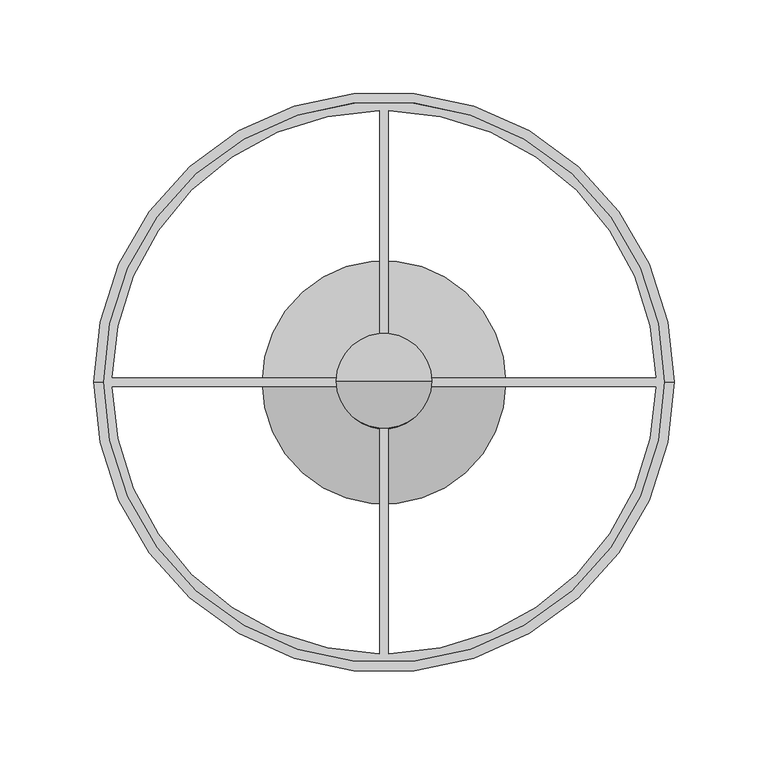
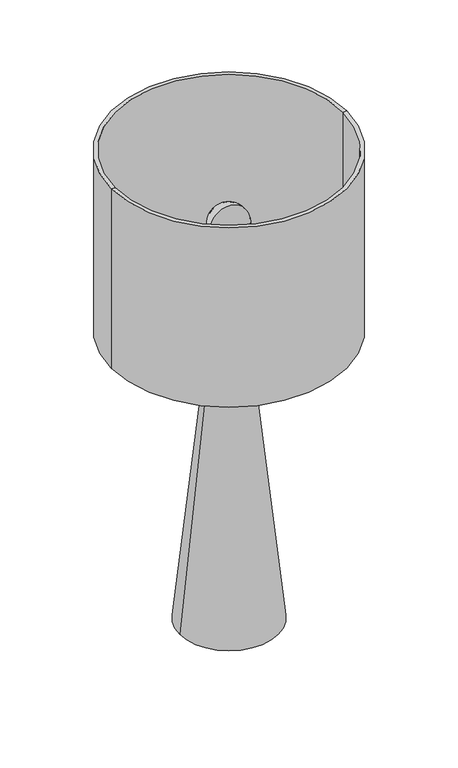
"""IFC4 building model written with IfcOpenShell, lengths in millimetres: furniture geometry."""

from ifc_helpers import new_model, si_unit, point, frame, frame_2d, origin, place, context, project, spatial, polyline, circle_curve, ellipse_curve, trimmed, segment, composite_curve, outline, extrude, source, transform, mapped, element, save
from ifc_brep_helpers import plane_surface, cylinder_surface, revolved_surface, advanced_brep


def furniture_2a5d2cbe(model_context):
    return source(origin(), model_context, "Body", "SolidModel", [
        advanced_brep(
        [(239.3621376, 642.8775263, 489.7915015), (258.4121376, 642.8775263, 489.7915015), (258.4121376, 642.8775263, 478.3555771), (239.3621376, 642.8775263, 478.3555771), (248.8871376, 642.8775263, 489.7915015), (245.7708139, 642.8775263, 472.622676), (252.0034612, 642.8775263, 472.622676), (248.8871376, 642.8775263, 472.622676), (244.5637531, 642.8775263, 474.7133667), (253.2105221, 642.8775263, 474.7133667)],
        [
            (0, 1, circle_curve(frame((248.8871376, 642.8775263, 489.7915015), z_axis=(0.0, 0.0, -1.0), x_axis=(1.0, 0.0, 0.0)), 9.525)),
            (1, 2),
            (2, 3, circle_curve(frame((248.8871376, 642.8775263, 478.3555771), z_axis=(0.0, 0.0, 1.0), x_axis=(1.0, 0.0, 0.0)), 9.525)),
            (3, 0),
            (1, 0, circle_curve(frame((248.8871376, 642.8775263, 489.7915015), z_axis=(0.0, 0.0, -1.0), x_axis=(1.0, 0.0, 0.0)), 9.525)),
            (3, 2, circle_curve(frame((248.8871376, 642.8775263, 478.3555771), z_axis=(0.0, 0.0, 1.0), x_axis=(1.0, 0.0, 0.0)), 9.525)),
            (4, 1),
            (0, 4),
            (5, 6, circle_curve(frame((248.8871376, 642.8775263, 472.622676), z_axis=(0.0, 0.0, -1.0), x_axis=(1.0, 0.0, 0.0)), 3.1163237)),
            (6, 7),
            (7, 5),
            (6, 5, circle_curve(frame((248.8871376, 642.8775263, 472.622676), z_axis=(0.0, 0.0, -1.0), x_axis=(1.0, 0.0, 0.0)), 3.1163237)),
            (8, 9, circle_curve(frame((248.8871376, 642.8775263, 474.7133667), z_axis=(0.0, 0.0, -1.0), x_axis=(1.0, 0.0, 0.0)), 4.3233845)),
            (9, 6),
            (5, 8),
            (9, 8, circle_curve(frame((248.8871376, 642.8775263, 474.7133667), z_axis=(0.0, 0.0, -1.0), x_axis=(1.0, 0.0, 0.0)), 4.3233845)),
            (2, 9),
            (8, 3),
        ],
        [
            cylinder_surface(frame((248.8871376, 642.8775263, 3081.6807772), z_axis=(0.0, 0.0, 1.0), x_axis=(1.0, 0.0, 0.0)), 9.525),
            plane_surface(frame((248.8871376, 642.8775263, 489.7915015), z_axis=(0.0, 0.0, 1.0), x_axis=(1.0, 0.0, 0.0))),
            plane_surface(frame((248.8871376, 642.8775263, 472.622676), z_axis=(0.0, 0.0, -1.0), x_axis=(1.0, 0.0, 0.0))),
            revolved_surface(polyline([(252.0034612, 642.8775263, 472.622676), (253.2105221, 642.8775263, 474.7133667)]), (248.8871376, 642.8775263, 3081.6807772), (0.0, 0.0, 1.0)),
            revolved_surface(polyline([(253.2105221, 642.8775263, 474.7133667), (258.4121376, 642.8775263, 478.3555771)]), (248.8871376, 642.8775263, 3081.6807772), (0.0, 0.0, 1.0)),
        ],
        [
            (0, [[1, 2, 3, 4]]),
            (0, [[5, -4, 6, -2]]),
            (1, [[7, -1, 8]]),
            (1, [[-8, -5, -7]]),
            (2, [[9, 10, 11]]),
            (2, [[12, -11, -10]]),
            (3, [[13, 14, -9, 15]]),
            (3, [[16, -15, -12, -14]]),
            (4, [[-3, 17, -13, 18]]),
            (4, [[-6, -18, -16, -17]]),
        ],
    ),
        advanced_brep(
        [(227.7699798, 642.8775263, 536.1920313), (270.0042954, 642.8775263, 536.1920313), (248.8871376, 642.8775263, 573.428926), (240.1558876, 642.8775263, 489.7915015), (257.6183876, 642.8775263, 489.7915015), (257.6183876, 642.8775263, 491.3545803), (240.1558876, 642.8775263, 491.3545803), (239.3621376, 642.8775263, 489.7915015), (258.4121376, 642.8775263, 489.7915015), (239.3621376, 642.8775263, 491.3545803), (258.4121376, 642.8775263, 491.3545803), (248.8871376, 642.8775263, 574.222676), (270.685494, 642.8775263, 535.7845911), (227.0887811, 642.8775263, 535.7845911)],
        [
            (0, 1, circle_curve(frame((248.8871376, 642.8775263, 536.1920313), z_axis=(0.0, 0.0, -1.0), x_axis=(1.0, 0.0, 0.0)), 21.1171578)),
            (1, 2, circle_curve(frame((248.8871376, 642.8775263, 548.822676), z_axis=(0.0, -1.0, 0.0), x_axis=(1.0, 0.0, 0.0)), 24.60625)),
            (2, 0, circle_curve(frame((248.8871376, 642.8775263, 548.822676), z_axis=(0.0, -1.0, 0.0), x_axis=(-1.0, 0.0, 0.0)), 24.60625)),
            (1, 0, circle_curve(frame((248.8871376, 642.8775263, 536.1920313), z_axis=(0.0, 0.0, -1.0), x_axis=(1.0, 0.0, 0.0)), 21.1171578)),
            (3, 4, circle_curve(frame((248.8871376, 642.8775263, 489.7915015), z_axis=(0.0, 0.0, -1.0), x_axis=(1.0, 0.0, 0.0)), 8.73125)),
            (4, 5),
            (5, 6, circle_curve(frame((248.8871376, 642.8775263, 491.3545803), z_axis=(0.0, 0.0, 1.0), x_axis=(1.0, 0.0, 0.0)), 8.73125)),
            (6, 3),
            (4, 3, circle_curve(frame((248.8871376, 642.8775263, 489.7915015), z_axis=(0.0, 0.0, -1.0), x_axis=(1.0, 0.0, 0.0)), 8.73125)),
            (6, 5, circle_curve(frame((248.8871376, 642.8775263, 491.3545803), z_axis=(0.0, 0.0, 1.0), x_axis=(1.0, 0.0, 0.0)), 8.73125)),
            (7, 8, circle_curve(frame((248.8871376, 642.8775263, 489.7915015), z_axis=(0.0, 0.0, -1.0), x_axis=(1.0, 0.0, 0.0)), 9.525)),
            (8, 4),
            (3, 7),
            (8, 7, circle_curve(frame((248.8871376, 642.8775263, 489.7915015), z_axis=(0.0, 0.0, -1.0), x_axis=(1.0, 0.0, 0.0)), 9.525)),
            (9, 10, circle_curve(frame((248.8871376, 642.8775263, 491.3545803), z_axis=(0.0, 0.0, -1.0), x_axis=(1.0, 0.0, 0.0)), 9.525)),
            (10, 8),
            (7, 9),
            (10, 9, circle_curve(frame((248.8871376, 642.8775263, 491.3545803), z_axis=(0.0, 0.0, -1.0), x_axis=(1.0, 0.0, 0.0)), 9.525)),
            (11, 12, circle_curve(frame((248.8871376, 642.8775263, 548.822676), z_axis=(0.0, 1.0, 0.0), x_axis=(1.0, 0.0, 0.0)), 25.4)),
            (12, 13, circle_curve(frame((248.8871376, 642.8775263, 535.7845911), z_axis=(0.0, 0.0, 1.0), x_axis=(1.0, 0.0, 0.0)), 21.7983564)),
            (13, 11, circle_curve(frame((248.8871376, 642.8775263, 548.822676), z_axis=(0.0, 1.0, 0.0), x_axis=(-1.0, 0.0, 0.0)), 25.4)),
            (13, 12, circle_curve(frame((248.8871376, 642.8775263, 535.7845911), z_axis=(0.0, 0.0, 1.0), x_axis=(1.0, 0.0, 0.0)), 21.7983564)),
            (5, 1, circle_curve(frame((344.9679691, 642.8775263, 491.3545803), z_axis=(0.0, 1.0, 0.0), x_axis=(1.0, 0.0, 0.0)), 87.3495815)),
            (0, 6, circle_curve(frame((152.8063061, 642.8775263, 491.3545803), z_axis=(0.0, 1.0, 0.0), x_axis=(-1.0, 0.0, 0.0)), 87.3495815)),
            (12, 10, circle_curve(frame((344.9679691, 642.8775263, 491.3545803), z_axis=(0.0, -1.0, 0.0), x_axis=(1.0, 0.0, 0.0)), 86.5558315)),
            (9, 13, circle_curve(frame((152.8063061, 642.8775263, 491.3545803), z_axis=(0.0, -1.0, 0.0), x_axis=(-1.0, 0.0, 0.0)), 86.5558315)),
        ],
        [
            revolved_surface(trimmed(ellipse_curve(frame((248.8871376, 642.8775263, 548.822676), z_axis=(0.0, 1.0, 0.0), x_axis=(1.0, 0.0, 0.0)), 24.60625, 24.60625), [point((248.8871376, 642.8775263, 573.428926))], [point((270.0042954, 642.8775263, 536.1920313))], True, "CARTESIAN"), (248.8871376, 642.8775263, 3081.6807772), (0.0, 0.0, 1.0)),
            revolved_surface(polyline([(257.6183876, 642.8775263, 491.3545803000002), (257.6183876, 642.8775263, 489.79150149999987)]), (248.8871376, 642.8775263, 3081.6807772), (0.0, 0.0, 1.0)),
            plane_surface(frame((248.8871376, 642.8775263, 489.7915015), z_axis=(0.0, 0.0, -1.0), x_axis=(1.0, 0.0, 0.0))),
            cylinder_surface(frame((248.8871376, 642.8775263, 3081.6807772), z_axis=(0.0, 0.0, 1.0), x_axis=(1.0, 0.0, 0.0)), 9.525),
            revolved_surface(trimmed(ellipse_curve(frame((248.8871376, 642.8775263, 548.822676), z_axis=(0.0, -1.0, 0.0), x_axis=(1.0, 0.0, 0.0)), 25.4, 25.4), [point((270.685494, 642.8775263, 535.7845911))], [point((248.8871376, 642.8775263, 574.222676))], True, "CARTESIAN"), (248.8871376, 642.8775263, 3081.6807772), (0.0, 0.0, 1.0)),
            revolved_surface(trimmed(ellipse_curve(frame((344.9679691, 642.8775263, 491.3545803), z_axis=(0.0, -1.0, 0.0), x_axis=(1.0, 0.0, 0.0)), 87.3495815, 87.3495815), [point((270.0042954, 642.8775263, 536.1920313))], [point((257.6183876, 642.8775263, 491.3545803))], True, "CARTESIAN"), (248.8871376, 642.8775263, 3081.6807772), (0.0, 0.0, 1.0)),
            revolved_surface(trimmed(ellipse_curve(frame((344.9679691, 642.8775263, 491.3545803), z_axis=(0.0, 1.0, 0.0), x_axis=(1.0, 0.0, 0.0)), 86.5558315, 86.5558315), [point((258.4121376, 642.8775263, 491.3545803))], [point((270.685494, 642.8775263, 535.7845911))], True, "CARTESIAN"), (248.8871376, 642.8775263, 3081.6807772), (0.0, 0.0, 1.0)),
        ],
        [
            (0, [[1, 2, 3]]),
            (0, [[4, -3, -2]]),
            (1, [[5, 6, 7, 8]]),
            (1, [[9, -8, 10, -6]]),
            (2, [[11, 12, -5, 13]]),
            (2, [[14, -13, -9, -12]]),
            (3, [[15, 16, -11, 17]]),
            (3, [[18, -17, -14, -16]]),
            (4, [[19, 20, 21]]),
            (4, [[-21, 22, -19]]),
            (5, [[-7, 23, -1, 24]]),
            (5, [[-10, -24, -4, -23]]),
            (6, [[-20, 25, -15, 26]]),
            (6, [[-22, -26, -18, -25]]),
        ],
    ),
        advanced_brep(
        [(183.8871376, 642.2035969, 0.0), (313.8871376, 642.2035969, 0.0), (248.8871376, 642.2035969, 0.0), (235.7140606, 642.2035969, 490.0), (262.0602145, 642.2035969, 490.0), (248.8871376, 642.2035969, 490.0)],
        [
            (0, 1, circle_curve(frame((248.8871376, 642.2035969, 0.0), z_axis=(0.0, 0.0, -1.0), x_axis=(1.0, 0.0, 0.0)), 65.0)),
            (1, 2),
            (2, 0),
            (1, 0, circle_curve(frame((248.8871376, 642.2035969, 0.0), z_axis=(0.0, 0.0, -1.0), x_axis=(1.0, 0.0, 0.0)), 65.0)),
            (3, 4, circle_curve(frame((248.8871376, 642.2035969, 490.0), z_axis=(0.0, 0.0, -1.0), x_axis=(1.0, 0.0, 0.0)), 13.1730769)),
            (4, 1),
            (0, 3),
            (4, 3, circle_curve(frame((248.8871376, 642.2035969, 490.0), z_axis=(0.0, 0.0, -1.0), x_axis=(1.0, 0.0, 0.0)), 13.1730769)),
            (5, 4),
            (3, 5),
        ],
        [
            plane_surface(frame((248.8871376, 642.2035969, 0.0), z_axis=(0.0, 0.0, -1.0), x_axis=(1.0, 0.0, 0.0))),
            revolved_surface(polyline([(313.8871376, 642.2035969, 0.0), (262.0602145, 642.2035969, 490.0)]), (248.8871376, 642.2035969, 0.0), (0.0, 0.0, 1.0)),
            plane_surface(frame((248.8871376, 642.2035969, 490.0), z_axis=(0.0, 0.0, 1.0), x_axis=(1.0, 0.0, 0.0))),
        ],
        [
            (0, [[1, 2, 3]]),
            (0, [[4, -3, -2]]),
            (1, [[5, 6, -1, 7]]),
            (1, [[8, -7, -4, -6]]),
            (2, [[9, -5, 10]]),
            (2, [[-10, -8, -9]]),
        ],
    ),
        advanced_brep(
        [(98.8871376, 642.2035969, 652.3668776), (398.8871376, 642.2035969, 652.3668776), (403.8871376, 642.2035969, 652.3668776), (93.8871376, 642.2035969, 652.3668776), (98.8871376, 642.2035969, 402.3668776), (398.8871376, 642.2035969, 402.3668776), (93.8871376, 642.2035969, 402.3668776), (403.8871376, 642.2035969, 402.3668776)],
        [
            (0, 1, circle_curve(frame((248.8871376, 642.2035969, 652.3668776), z_axis=(0.0, 0.0, -1.0), x_axis=(1.0, 0.0, 0.0)), 150.0)),
            (1, 2),
            (2, 3, circle_curve(frame((248.8871376, 642.2035969, 652.3668776), z_axis=(0.0, 0.0, 1.0), x_axis=(1.0, 0.0, 0.0)), 155.0)),
            (3, 0),
            (1, 0, circle_curve(frame((248.8871376, 642.2035969, 652.3668776), z_axis=(0.0, 0.0, -1.0), x_axis=(1.0, 0.0, 0.0)), 150.0)),
            (3, 2, circle_curve(frame((248.8871376, 642.2035969, 652.3668776), z_axis=(0.0, 0.0, 1.0), x_axis=(1.0, 0.0, 0.0)), 155.0)),
            (4, 5, circle_curve(frame((248.8871376, 642.2035969, 402.3668776), z_axis=(0.0, 0.0, -1.0), x_axis=(1.0, 0.0, 0.0)), 150.0)),
            (5, 1),
            (0, 4),
            (5, 4, circle_curve(frame((248.8871376, 642.2035969, 402.3668776), z_axis=(0.0, 0.0, -1.0), x_axis=(1.0, 0.0, 0.0)), 150.0)),
            (6, 7, circle_curve(frame((248.8871376, 642.2035969, 402.3668776), z_axis=(0.0, 0.0, -1.0), x_axis=(1.0, 0.0, 0.0)), 155.0)),
            (7, 5),
            (4, 6),
            (7, 6, circle_curve(frame((248.8871376, 642.2035969, 402.3668776), z_axis=(0.0, 0.0, -1.0), x_axis=(1.0, 0.0, 0.0)), 155.0)),
            (2, 7),
            (6, 3),
        ],
        [
            plane_surface(frame((248.8871376, 642.2035969, 652.3668776), z_axis=(0.0, 0.0, 1.0), x_axis=(1.0, 0.0, 0.0))),
            revolved_surface(polyline([(398.88713759999996, 642.2035969, 652.3668776), (398.88713759999996, 642.2035969, 402.3668776)]), (248.8871376, 642.2035969, 652.3668776), (0.0, 0.0, 1.0)),
            plane_surface(frame((248.8871376, 642.2035969, 402.3668776), z_axis=(0.0, 0.0, -1.0), x_axis=(1.0, 0.0, 0.0))),
            cylinder_surface(frame((248.8871376, 642.2035969, 652.3668776), z_axis=(0.0, 0.0, 1.0), x_axis=(1.0, 0.0, 0.0)), 155.0),
        ],
        [
            (0, [[1, 2, 3, 4]]),
            (0, [[5, -4, 6, -2]]),
            (1, [[7, 8, -1, 9]]),
            (1, [[10, -9, -5, -8]]),
            (2, [[11, 12, -7, 13]]),
            (2, [[14, -13, -10, -12]]),
            (3, [[-3, 15, -11, 16]]),
            (3, [[-6, -16, -14, -15]]),
        ],
    ),
        extrude(outline(composite_curve([segment(trimmed(circle_curve(frame_2d((248.8871376, 642.2035969)), 150.0), [point((98.8871376, 642.2035969))], [point((398.8871376, 642.2035969))], False, "CARTESIAN"), True, "CONTINUOUS"), segment(trimmed(circle_curve(frame_2d((248.8871376, 642.2035969)), 150.0), [point((398.8871376, 642.2035969))], [point((98.8871376, 642.2035969))], False, "CARTESIAN"), True, "CONTINUOUS")], self_intersect=False), holes=[composite_curve([segment(polyline([(251.3871376, 787.1820436), (251.3871376, 667.0782829)]), True, "CONTINUOUS"), segment(trimmed(circle_curve(frame_2d((248.8871376, 642.2035969)), 25.0), [point((251.3871376, 667.0782829))], [point((273.7618235, 644.7035969))], False, "CARTESIAN"), True, "CONTINUOUS"), segment(polyline([(273.7618235, 644.7035969), (393.8655842, 644.7035969)]), True, "CONTINUOUS"), segment(trimmed(circle_curve(frame_2d((248.8871376, 642.2035969)), 145.0), [point((393.8655842, 644.7035969))], [point((251.3871376, 787.1820436))], True, "CARTESIAN"), True, "CONTINUOUS")], self_intersect=False), composite_curve([segment(polyline([(246.3871376, 497.2251503), (246.3871376, 617.328911)]), True, "CONTINUOUS"), segment(trimmed(circle_curve(frame_2d((248.8871376, 642.2035969)), 25.0), [point((246.3871376, 617.328911))], [point((224.0124516, 639.7035969))], False, "CARTESIAN"), True, "CONTINUOUS"), segment(polyline([(224.0124516, 639.7035969), (103.9086909, 639.7035969)]), True, "CONTINUOUS"), segment(trimmed(circle_curve(frame_2d((248.8871376, 642.2035969)), 145.0), [point((103.9086909, 639.7035969))], [point((246.3871376, 497.2251503))], True, "CARTESIAN"), True, "CONTINUOUS")], self_intersect=False), composite_curve([segment(polyline([(246.3871376, 667.0782829), (246.3871376, 787.1820436)]), True, "CONTINUOUS"), segment(trimmed(circle_curve(frame_2d((248.8871376, 642.2035969)), 145.0), [point((246.3871376, 787.1820436))], [point((103.9086909, 644.7035969))], True, "CARTESIAN"), True, "CONTINUOUS"), segment(polyline([(103.9086909, 644.7035969), (224.0124516, 644.7035969)]), True, "CONTINUOUS"), segment(trimmed(circle_curve(frame_2d((248.8871376, 642.2035969)), 25.0), [point((224.0124516, 644.7035969))], [point((246.3871376, 667.0782829))], False, "CARTESIAN"), True, "CONTINUOUS")], self_intersect=False), composite_curve([segment(polyline([(393.8655842, 639.7035969), (273.7618235, 639.7035969)]), True, "CONTINUOUS"), segment(trimmed(circle_curve(frame_2d((248.8871376, 642.2035969)), 25.0), [point((273.7618235, 639.7035969))], [point((251.3871376, 617.328911))], False, "CARTESIAN"), True, "CONTINUOUS"), segment(polyline([(251.3871376, 617.328911), (251.3871376, 497.2251503)]), True, "CONTINUOUS"), segment(trimmed(circle_curve(frame_2d((248.8871376, 642.2035969)), 145.0), [point((251.3871376, 497.2251503))], [point((393.8655842, 639.7035969))], True, "CARTESIAN"), True, "CONTINUOUS")], self_intersect=False), composite_curve([segment(trimmed(circle_curve(frame_2d((248.8871376, 642.2035969)), 20.0), [point((248.7275476, 662.2029602))], [point((228.8871376, 642.2035969))], True, "CARTESIAN"), True, "CONTINUOUS"), segment(trimmed(circle_curve(frame_2d((248.8871376, 642.2035969)), 20.0), [point((228.8871376, 642.2035969))], [point((268.8871376, 642.2035969))], True, "CARTESIAN"), True, "CONTINUOUS"), segment(trimmed(circle_curve(frame_2d((248.8871376, 642.2035969)), 20.0), [point((268.8871376, 642.2035969))], [point((248.7275476, 662.2029602))], True, "CARTESIAN"), True, "CONTINUOUS")], self_intersect=False)]), frame((0.0, 0.0, 440.0), z_axis=(0.0, 0.0, 1.0), x_axis=(1.0, 0.0, 0.0)), (0.0, 0.0, 1.0), 5.0),
    ])


if __name__ == "__main__":
    model = new_model("IFC4")
    model_context = context("Model", 3, world=origin())
    ifc_project = project(units=[si_unit("LENGTHUNIT", "METRE", prefix="MILLI")], contexts=[model_context])
    site = spatial("IfcSite", under=ifc_project)
    building = spatial("IfcBuilding", under=site)
    placement = place(None, origin())
    furniture_shape = furniture_2a5d2cbe(model_context)
    element("IfcFurniture", 1, at=placement, inside=building, context=model_context, shape_type="MappedRepresentation", body=[
        mapped(furniture_shape, transform((0.0, 0.0, 0.0), x_axis=(1.0, 0.0, 0.0), y_axis=(0.0, 1.0, 0.0), z_axis=(0.0, 0.0, 1.0))),
    ])
    save(model, "model.ifc")

# Revit data of these elements
# Type
#   Default Elevation = 0
# Element 1 (IfcFurniture)
#   Materials on its faces: "Metal - Chrome Polished"
# Materials
#   "Metal - Chrome Polished": class "Metal", colour RGB 247 247 247, transparency 0
